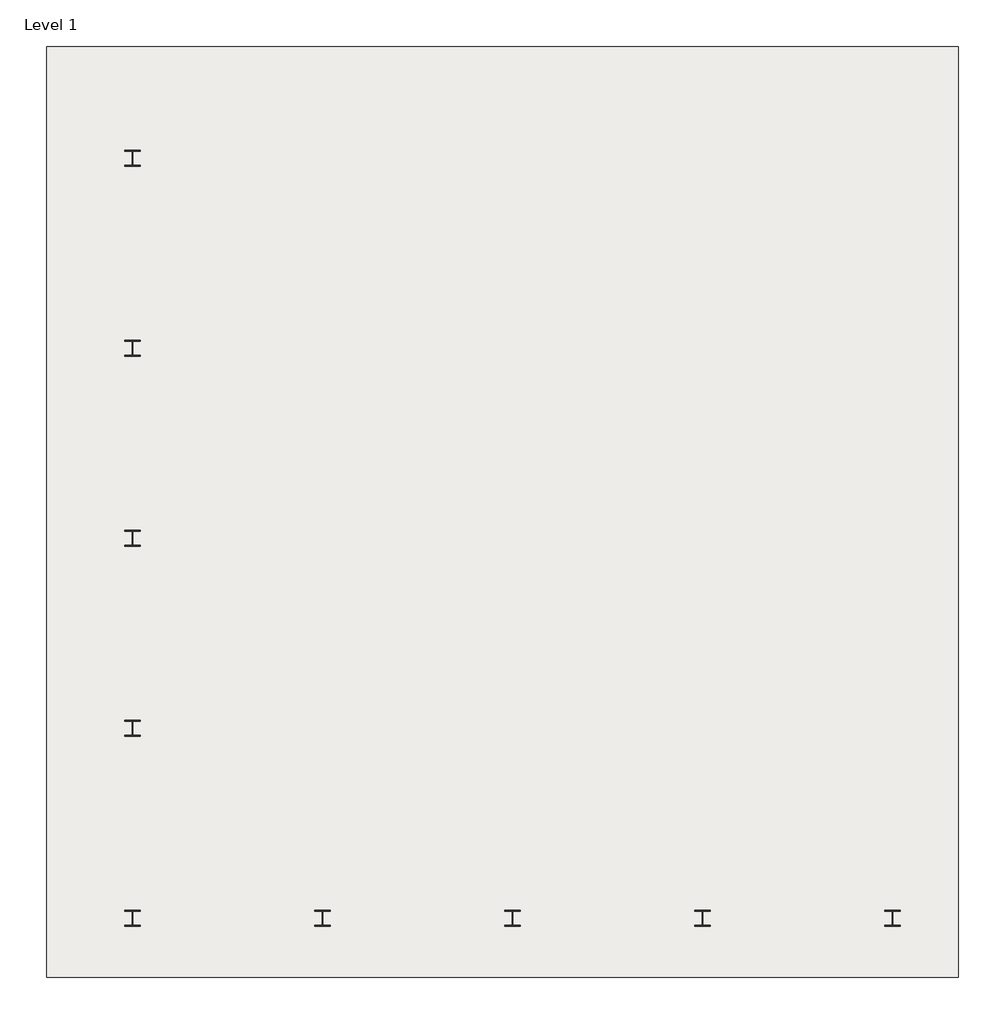
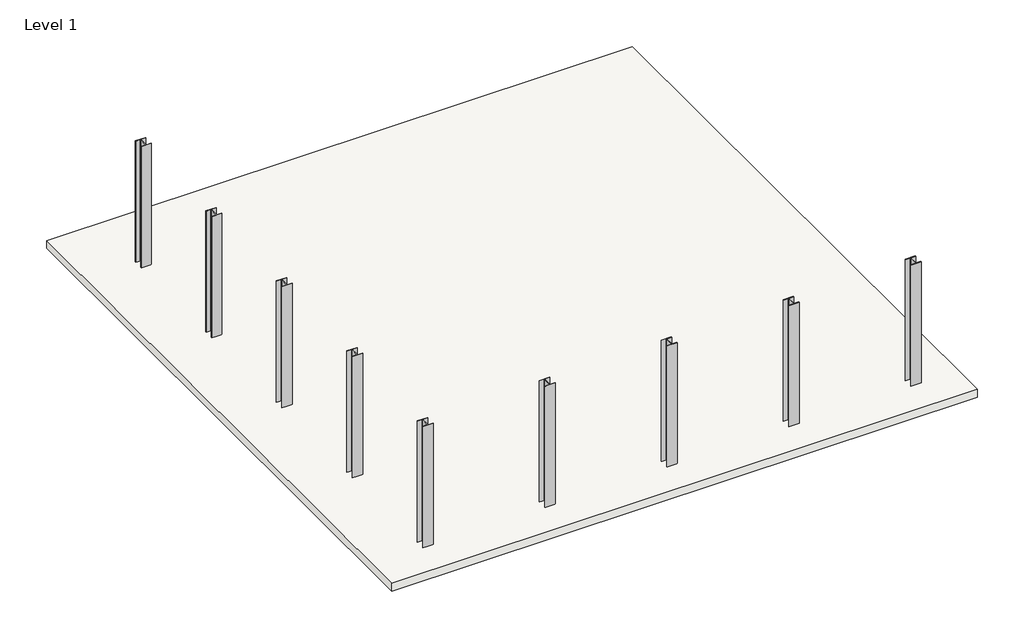
# One storey: 9 columns, 1 slab.
"""IFC4 building model written with IfcOpenShell, lengths in millimetres."""

from ifc_helpers import new_model, si_unit, frame, origin, place, context, project, spatial, polyline, outline, extrude, transform, mapped, element, save
from components import w_shapes_column_w10x49_27dd9c5e

model = new_model("IFC4")

# Units and contexts
model_context = context("Model", 3, world=origin())
ifc_project = project(units=[si_unit("LENGTHUNIT", "METRE", prefix="MILLI")], contexts=[model_context])

# Site, building, storey
site = spatial("IfcSite", under=ifc_project)
building = spatial("IfcBuilding", under=site)
storey = spatial("IfcBuildingStorey", under=building, Name="Level 1", Elevation=0.0)

# Columns
placement = place(None, origin())
w_shapes_column_w10x49_shape = w_shapes_column_w10x49_27dd9c5e(model_context)
element("IfcColumn", 1, ObjectType="W Shapes-Column : W10X49", at=placement, inside=storey, context=model_context, shape_type="MappedRepresentation", body=[
    mapped(w_shapes_column_w10x49_shape, transform((-17802.1103918, -9032.5390156, 0.0), x_axis=(1.0, 0.0, 0.0), y_axis=(0.0, 1.0, 0.0), z_axis=(0.0, 0.0, 1.0))),
])
element("IfcColumn", 2, ObjectType="W Shapes-Column : W10X49", at=placement, inside=storey, context=model_context, shape_type="MappedRepresentation", body=[
    mapped(w_shapes_column_w10x49_shape, transform((-14754.1103918, -9032.5390156, 0.0), x_axis=(1.0, 0.0, 0.0), y_axis=(0.0, 1.0, 0.0), z_axis=(0.0, 0.0, 1.0))),
])
element("IfcColumn", 3, ObjectType="W Shapes-Column : W10X49", at=placement, inside=storey, context=model_context, shape_type="MappedRepresentation", body=[
    mapped(w_shapes_column_w10x49_shape, transform((-11706.1103918, -9032.5390156, 0.0), x_axis=(1.0, 0.0, 0.0), y_axis=(0.0, 1.0, 0.0), z_axis=(0.0, 0.0, 1.0))),
])
element("IfcColumn", 4, ObjectType="W Shapes-Column : W10X49", at=placement, inside=storey, context=model_context, shape_type="MappedRepresentation", body=[
    mapped(w_shapes_column_w10x49_shape, transform((-8658.1103918, -9032.5390156, 0.0), x_axis=(1.0, 0.0, 0.0), y_axis=(0.0, 1.0, 0.0), z_axis=(0.0, 0.0, 1.0))),
])
element("IfcColumn", 5, ObjectType="W Shapes-Column : W10X49", at=placement, inside=storey, context=model_context, shape_type="MappedRepresentation", body=[
    mapped(w_shapes_column_w10x49_shape, transform((-5610.1103918, -9032.5390156, 0.0), x_axis=(1.0, 0.0, 0.0), y_axis=(0.0, 1.0, 0.0), z_axis=(0.0, 0.0, 1.0))),
])
element("IfcColumn", 6, ObjectType="W Shapes-Column : W10X49", at=placement, inside=storey, context=model_context, shape_type="MappedRepresentation", body=[
    mapped(w_shapes_column_w10x49_shape, transform((-17802.1103918, -5984.5390156, 0.0), x_axis=(1.0, 0.0, 0.0), y_axis=(0.0, 1.0, 0.0), z_axis=(0.0, 0.0, 1.0))),
])
element("IfcColumn", 7, ObjectType="W Shapes-Column : W10X49", at=placement, inside=storey, context=model_context, shape_type="MappedRepresentation", body=[
    mapped(w_shapes_column_w10x49_shape, transform((-17802.1103918, -2936.5390156, 0.0), x_axis=(1.0, 0.0, 0.0), y_axis=(0.0, 1.0, 0.0), z_axis=(0.0, 0.0, 1.0))),
])
element("IfcColumn", 8, ObjectType="W Shapes-Column : W10X49", at=placement, inside=storey, context=model_context, shape_type="MappedRepresentation", body=[
    mapped(w_shapes_column_w10x49_shape, transform((-17802.1103918, 111.4609844, 0.0), x_axis=(1.0, 0.0, 0.0), y_axis=(0.0, 1.0, 0.0), z_axis=(0.0, 0.0, 1.0))),
])
element("IfcColumn", 9, ObjectType="W Shapes-Column : W10X49", at=placement, inside=storey, context=model_context, shape_type="MappedRepresentation", body=[
    mapped(w_shapes_column_w10x49_shape, transform((-17802.1103918, 3159.4609844, 0.0), x_axis=(1.0, 0.0, 0.0), y_axis=(0.0, 1.0, 0.0), z_axis=(0.0, 0.0, 1.0))),
])

# Slab
element("IfcSlab", 10, ObjectType="Generic - 12\"", at=placement, inside=storey, context=model_context, shape_type="SweptSolid", body=[
    extrude(outline(polyline([(-4551.5296876, 4953.3940048), (-4551.5296876, -9981.8059952), (-19181.9296876, -9981.8059952), (-19181.9296876, 4953.3940048), (-4551.5296876, 4953.3940048)])), frame((0.0, 0.0, -203.2), z_axis=(0.0, 0.0, 1.0), x_axis=(1.0, 0.0, 0.0)), (0.0, 0.0, 1.0), 203.2),
])

save(model, "model.ifc")

# Revit data of these elements
# Type "W Shapes-Column : W10X49"
#   Section Name Key = "W10x49"
#   Assembly Code = "B10"
#   Width = 10.000"
#   Web Thickness = 0.340"
#   Web Fillet = 0.500"
#   Warping Constant = 2070.00 in⁶
#   Torsional Moment of Inertia = 1.39 in⁴
#   Section Area = 14.40 in²
#   Plastic Modulus weak axis = 28.30 in³
#   Plastic Modulus strong axis = 60.40 in³
#   Perimeter = 58.50 ft²/ft
#   Nominal Weight = 49.00 lbf/ft
#   Moment of Inertia weak axis = 93.40 in⁴
#   Moment of Inertia strong axis = 272.00 in⁴
#   Height = 10.000"
#   Flange Thickness = 0.560"
#   Elastic Modulus weak axis = 18.70 in³
#   Elastic Modulus strong axis = 54.60 in³
#   Centroid Vertical = 5.000"
#   Centroid Horizontal = 5.000"
#   Structural Material [instance default] = Steel ASTM A992
#   Principal Axes Angle = 0
# Type "Generic - 12\""
#   Assembly Code = "B1010"
#   Function = 0
#   Layers, outside or top first: 0' - 8" no material (function 1)
# Elements 1, 2, 3, 4, 5, 6, 7, 8, 9 (IfcColumn, "W Shapes-Column : W10X49")
#   Structural Material = Steel ASTM A992
#   Phase Created = New Construction
#   Materials on its faces: "Steel ASTM A992"
# Element 10 (IfcSlab, "Generic - 12\"")
#   Height Offset From Level = 0' - 0"
#   Phase Created = New Construction
#   Materials on its faces: "Default Floor"
# Materials
#   "Steel ASTM A992": class "Metal", colour RGB 199 199 199, transparency 0, Description = "Structural steel 50ksi", Cost = 0
#   "Default Floor": colour RGB 128 128 128, transparency 0
